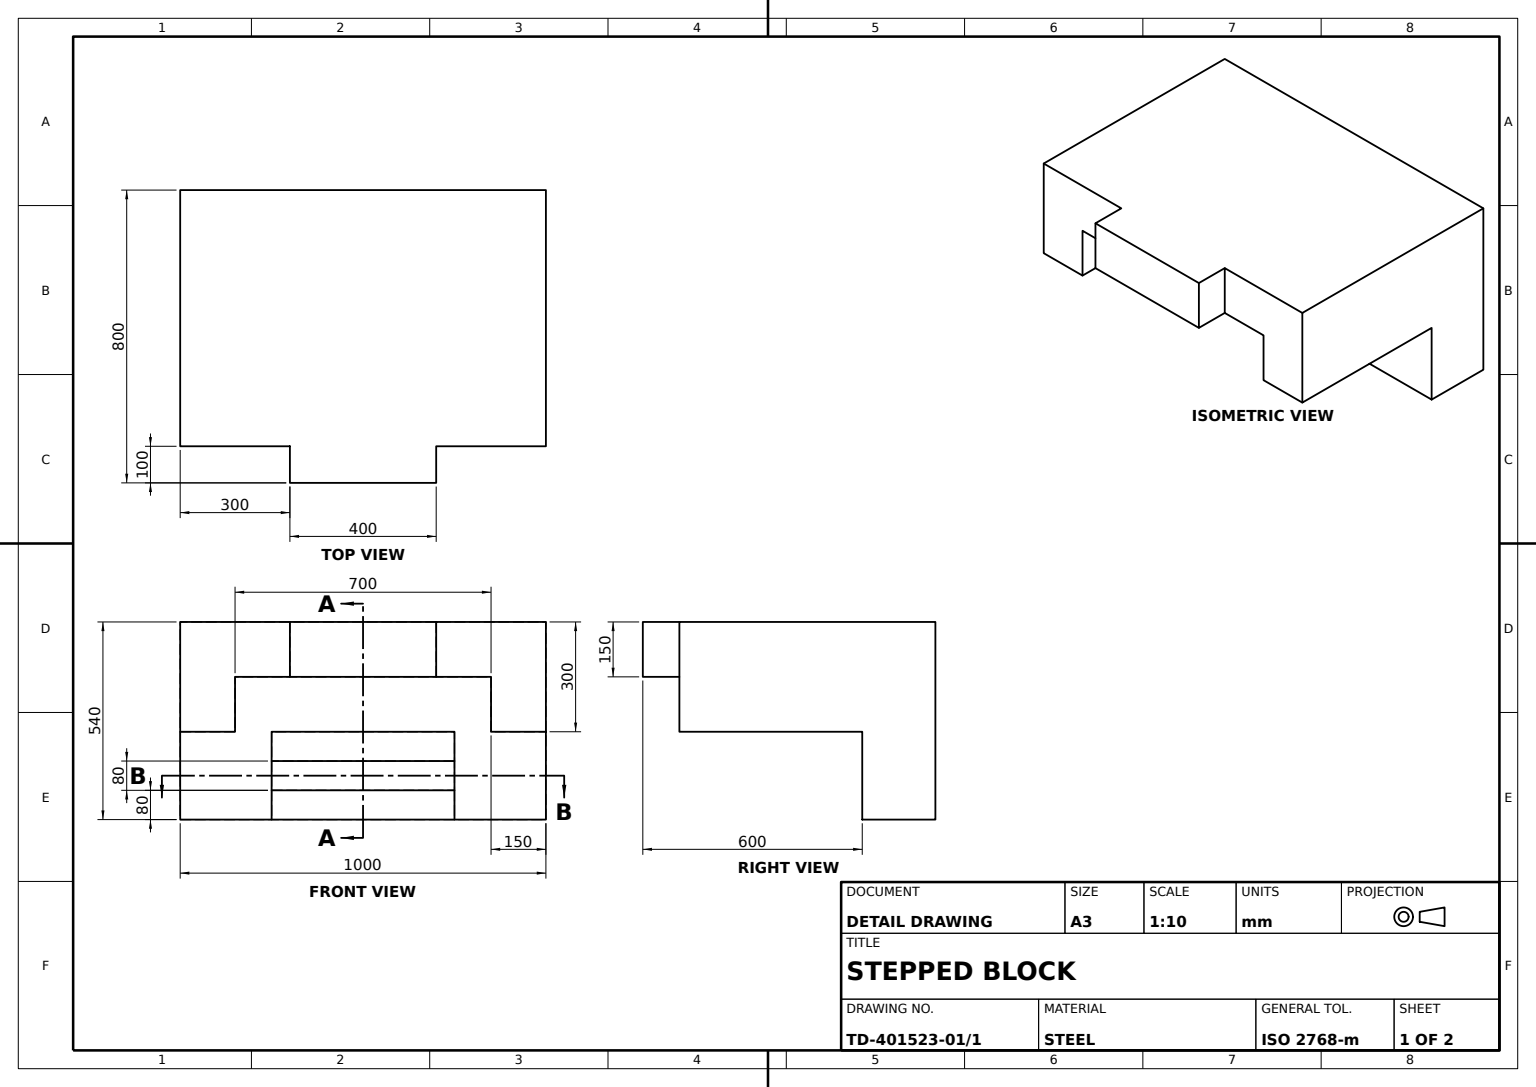
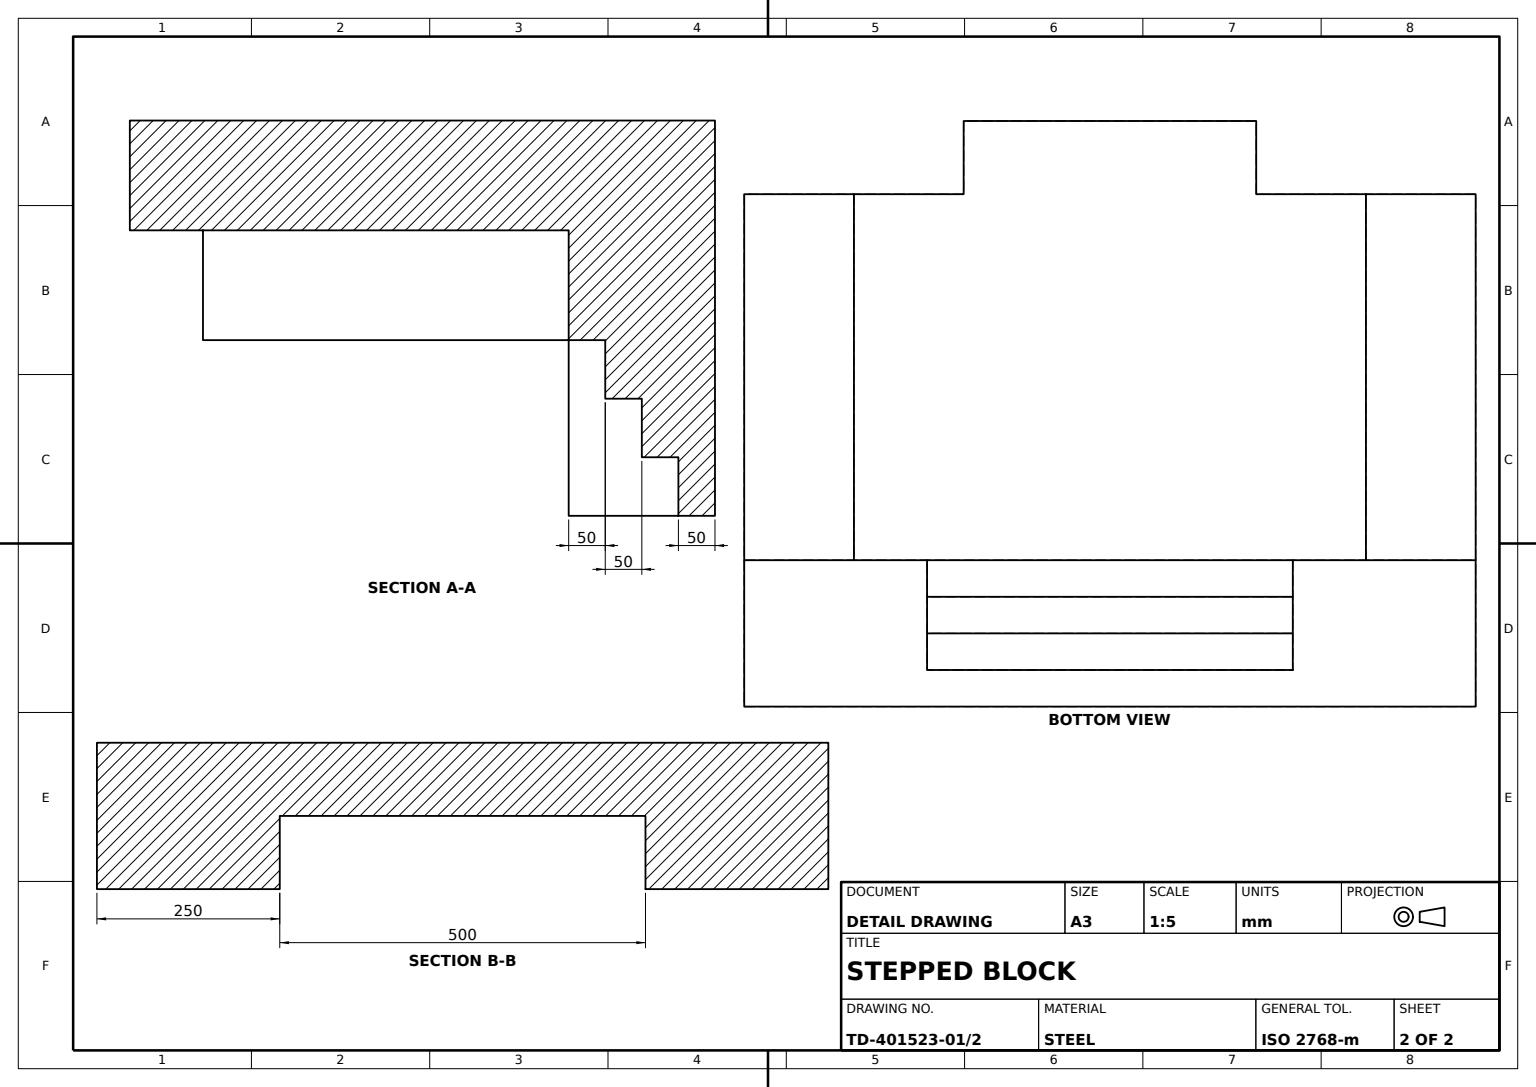
from build123d import *

# Parameters (mm, degrees)
BASE_BLOCK_PROFILE_W            = 1000
BASE_BLOCK_PROFILE_H            = 540
BASE_BLOCK_DEPTH                = 200
RAISED_BLOCK_PROFILE_W          = 600
RAISED_BLOCK_PROFILE_H          = 300
RAISED_BLOCK_DEPTH              = 1000
RAISED_BLOCK_STEP_CUT_PROFILE_W = 1000
RAISED_BLOCK_STEP_CUT_PROFILE_H = 300
RAISED_BLOCK_STEP_CUT_DEPTH     = 100
STAIR_STEP_BOSS_PROFILE_W       = 200
STAIR_STEP_BOSS_PROFILE_H       = 100
STAIR_STEP_BOSS_DEPTH           = 150
STAIR_CUTOUT_DEPTH              = 150
STEPPED_SLOT_PROFILE_W          = 250
STEPPED_SLOT_PROFILE_H          = 80
STEPPED_SLOT_CUT_DEPTH          = 150
SLOT_SECOND_STEP_PROFILE_W      = 500
SLOT_SECOND_STEP_PROFILE_H      = 80
SLOT_SECOND_STEP_CUT_DEPTH      = 100
SLOT_THIRD_STEP_PROFILE_W       = 500
SLOT_THIRD_STEP_PROFILE_H       = 80
SLOT_THIRD_STEP_CUT_DEPTH       = 50


with BuildPart() as part:
    # Base Block Profile → Base Block (new body)
    with BuildSketch(Plane.XY):
        with Locations((500, 270)):
            Rectangle(BASE_BLOCK_PROFILE_W, BASE_BLOCK_PROFILE_H)
    extrude(amount=BASE_BLOCK_DEPTH)

    # Raised Block Profile → Raised Block (add)
    with BuildSketch(Plane(origin=(1000, 0, 0), x_dir=(0, 0, -1), z_dir=(1, 0, 0))):
        with Locations((-500, 390)):
            Rectangle(RAISED_BLOCK_PROFILE_W, RAISED_BLOCK_PROFILE_H)
    extrude(amount=-RAISED_BLOCK_DEPTH)

    # Raised Block Step Cut Profile → Raised Block Step Cut (cut)
    with BuildSketch(Plane.XY.offset(800)):
        with Locations((500, 390)):
            Rectangle(RAISED_BLOCK_STEP_CUT_PROFILE_W, RAISED_BLOCK_STEP_CUT_PROFILE_H)
    extrude(amount=-RAISED_BLOCK_STEP_CUT_DEPTH, mode=Mode.SUBTRACT)

    # Stair Step Boss Profile → Stair Step Boss (add)
    with BuildSketch(Plane(origin=(0, 540, 0), x_dir=(1, 0, 0), z_dir=(0, 1, 0))):
        with Locations((400, -750)):
            Rectangle(STAIR_STEP_BOSS_PROFILE_W, STAIR_STEP_BOSS_PROFILE_H)
        with Locations((600, -750)):
            Rectangle(STAIR_STEP_BOSS_PROFILE_W, STAIR_STEP_BOSS_PROFILE_H)
    extrude(amount=-STAIR_STEP_BOSS_DEPTH)

    # Stair Cutout Profile → Stair Cutout (cut)
    with BuildSketch(Plane.XZ.offset(-240)):
        Polygon((500, 700), (150, 700), (150, 200), (850, 200), (850, 700), align=None)
    extrude(amount=-STAIR_CUTOUT_DEPTH, mode=Mode.SUBTRACT)

    # Stepped Slot Profile → Stepped Slot Cut (cut)
    with BuildSketch(Plane.XY.offset(200)):
        with Locations((375, 40)):
            Rectangle(STEPPED_SLOT_PROFILE_W, STEPPED_SLOT_PROFILE_H)
        with Locations((625, 40)):
            Rectangle(STEPPED_SLOT_PROFILE_W, STEPPED_SLOT_PROFILE_H)
    extrude(amount=-STEPPED_SLOT_CUT_DEPTH, mode=Mode.SUBTRACT)

    # Slot Second Step Profile → Slot Second Step Cut (cut)
    with BuildSketch(Plane.XY.offset(200)):
        with Locations((500, 120)):
            Rectangle(SLOT_SECOND_STEP_PROFILE_W, SLOT_SECOND_STEP_PROFILE_H)
    extrude(amount=-SLOT_SECOND_STEP_CUT_DEPTH, mode=Mode.SUBTRACT)

    # Slot Third Step Profile → Slot Third Step Cut (cut)
    with BuildSketch(Plane.XY.offset(200)):
        with Locations((500, 200)):
            Rectangle(SLOT_THIRD_STEP_PROFILE_W, SLOT_THIRD_STEP_PROFILE_H)
    extrude(amount=-SLOT_THIRD_STEP_CUT_DEPTH, mode=Mode.SUBTRACT)


solid = part.part
